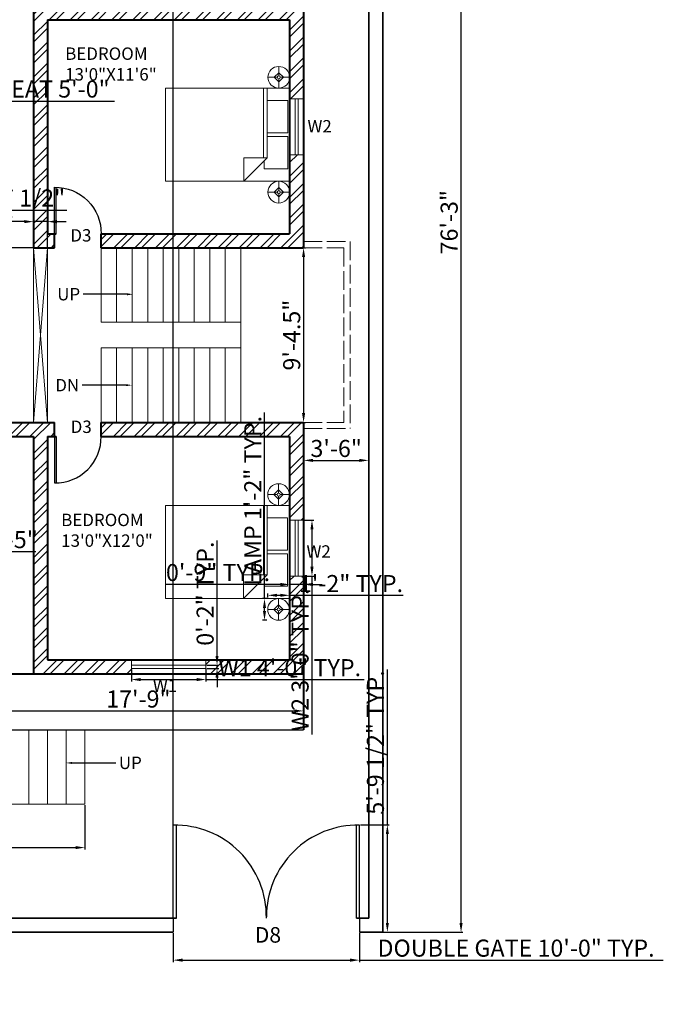
# Model space of a CAD drawing. Units: inches. Extents: x 2069 to 3028, y 691 to 1726.
# Tile 6 of 10: x 2613 to 3028, y 691 to 1325. Entities that reach past the tile are written whole.
import ezdxf
from ezdxf import colors
from ezdxf.entities.mleader import LeaderData, LeaderLine
from ezdxf.math import Vec2, Vec3

# ---------------------------------------------------------------- set-up
doc = ezdxf.new("R2010")
doc.units = ezdxf.units.IN
doc.linetypes.add('ACAD_ISO02W100', pattern=[15, 12, -3])
for name, color, linetype, lineweight in [('A-ANNO-DIMS', 2, 'Continuous', 18), ('A-DOOR', 3, 'Continuous', 25), ('A-FLOR', 7, 'Continuous', 25), ('A-FLOR-STRS', 7, 'Continuous', 20), ('A-FLOR-STRS-OVHD', 8, 'ACAD_ISO02W100', 18), ('A-FURN', 8, 'Continuous', 18), ('A-GLAZ', 4, 'Continuous', 20), ('A-WALL', 7, 'Continuous', 40), ('L-SITE-GATE', 3, 'Continuous', 25), ('L-SITE-WALL', 7, 'Continuous', 35)]:
    doc.layers.add(name, color=color, linetype=linetype, lineweight=lineweight)
for name, color, linetype, lineweight, true_color in [('A-ANNO-TEXT', 11, 'Continuous', 18, 0xf27172), ('A-AREA-IDEN', 11, 'Continuous', 25, 0xf27172), ('A-WALL-OPEN', 143, 'Continuous', 20, 0x7aafdf), ('A-WALL-PATT', 143, 'Continuous', 13, 0x7aafdf)]:
    doc.layers.add(name, color=color, linetype=linetype, lineweight=lineweight, true_color=true_color)
doc.styles.get("Standard").update_dxf_attribs({"font": 'arial.ttf'})
doc.dimstyles.new('ISO-25', dxfattribs={"dimtxt": 11, "dimasz": 6, "dimexe": 1.25, "dimexo": 0.625, "dimtad": 1, "dimlunit": 3, "dimtxsty": 'Standard', "dimcen": 2.5, "dimclrd": 3, "dimclre": 5, "dimclrt": 6, "dimadec": 0, "dimazin": 0, "dimtfac": 1, "dimtmove": 0, "dimatfit": 3, "dimfxl": 1, "dimarcsym": 0})

# ---------------------------------------------------------------- blocks, each defined once
blk = doc.blocks.new('Bed - Queen')
for p, q in [((0, -80.00003), (0, 0)), ((0, 0), (59.99999, 0)), ((59.99999, 0), (59.99999, -80.00003)), ((7.99999, -1.2), (28.79998, -1.2)), ((7.99999, -14.4), (7.99999, -1.2)), ((28.79998, -1.2), (28.79998, -14.4)), ((31.19999, -1.2), (51.99999, -1.2)), ((31.19999, -14.4), (31.19999, -1.2)), ((51.99999, -1.2), (51.99999, -16.4)), ((0, -14.4), (44.8, -14.4)), ((44.8, -16.8), (0, -16.8)), ((59.99999, -29.6), (44.8, -14.4)), ((44.8, -14.4), (44.8, -29.6)), ((51.99999, -16.4), (46.79936, -16.4)), ((44.8, -29.6), (59.99999, -29.6)), ((59.99999, -80.00003), (0, -80.00003))]:
    blk.add_line(p, q)
blk = doc.blocks.new('Lamp - Table')
for p, q in [((0, 7), (0, 1)), ((-1, 0), (-7, 0)), ((0, 3), (-3, 0)), ((-3, 0), (0, -3)), ((3, 0), (0, 3)), ((0, -3), (3, 0)), ((1, 0), (7, 0)), ((0, -1), (0, -7))]:
    blk.add_line(p, q)
for radius in [7, 1]:
    blk.add_circle((0, 0), radius)
blk = doc.blocks.new('*D26')
at = {"layer": 'A-ANNO-DIMS', "color": 0, "lineweight": -2, "transparency": 16777216}
for p, q in [((2796.58, 1178.39), (2797.2, 1178.39)), ((2795.95, 1172.39), (2795.95, 1071.89)), ((2796.58, 1065.89), (2797.2, 1065.89))]:
    blk.add_line(p, q, dxfattribs=at)
at = {"layer": 'A-ANNO-DIMS', "color": 0, "transparency": 16777216}
for points in [[(2794.95, 1172.39), (2796.95, 1172.39), (2795.95, 1178.39)], [(2794.95, 1071.89), (2796.95, 1071.89), (2795.95, 1065.89)]]:
    blk.add_solid(points, dxfattribs=at)
at = {"layer": 'Defpoints', "color": 0, "transparency": 16777216}
for p in [(2795.95, 1178.39), (2795.95, 1065.89), (2795.95, 1065.89)]:
    blk.add_point(p, dxfattribs=at)
at = {"layer": 'A-ANNO-DIMS', "color": 0, "transparency": 16777216, "insert": (2789.71, 1122.14), "char_height": 11, "attachment_point": 5, "rotation": 90}
blk.add_mtext('9\'-4.5"', dxfattribs=at)
blk = doc.blocks.new('*D27')
at = {"layer": 'A-ANNO-DIMS', "color": 0, "lineweight": -2, "transparency": 16777216}
for p, q in [((2795.95, 1060.76), (2795.95, 1040.17)), ((2837.95, 1060.76), (2837.95, 1040.17)), ((2801.95, 1041.42), (2831.95, 1041.42))]:
    blk.add_line(p, q, dxfattribs=at)
at = {"layer": 'A-ANNO-DIMS', "color": 0, "transparency": 16777216}
for points in [[(2801.95, 1042.42), (2801.95, 1040.42), (2795.95, 1041.42)], [(2831.95, 1042.42), (2831.95, 1040.42), (2837.95, 1041.42)]]:
    blk.add_solid(points, dxfattribs=at)
at = {"layer": 'Defpoints', "color": 0, "transparency": 16777216}
for p in [(2795.95, 1061.39), (2837.95, 1061.39), (2837.95, 1041.42)]:
    blk.add_point(p, dxfattribs=at)
at = {"layer": 'A-ANNO-DIMS', "color": 0, "transparency": 16777216, "insert": (2816.95, 1047.67), "char_height": 11, "attachment_point": 5}
blk.add_mtext('3\'-6"', dxfattribs=at)
blk = doc.blocks.new('*D28')
at = {"layer": 'A-ANNO-DIMS', "color": 0, "lineweight": -2, "transparency": 16777216}
for p, q in [((2582.95, 868.51), (2582.95, 881.23)), ((2588.95, 879.98), (2789.95, 879.98)), ((2795.95, 868.51), (2795.95, 881.23))]:
    blk.add_line(p, q, dxfattribs=at)
at = {"layer": 'A-ANNO-DIMS', "color": 0, "transparency": 16777216}
for points in [[(2588.95, 880.98), (2588.95, 878.98), (2582.95, 879.98)], [(2789.95, 880.98), (2789.95, 878.98), (2795.95, 879.98)]]:
    blk.add_solid(points, dxfattribs=at)
at = {"layer": 'Defpoints', "color": 0, "transparency": 16777216}
for p in [(2795.95, 879.98), (2582.95, 867.89), (2795.95, 867.89)]:
    blk.add_point(p, dxfattribs=at)
at = {"layer": 'A-ANNO-DIMS', "color": 0, "transparency": 16777216, "insert": (2689.45, 886.22), "char_height": 11, "attachment_point": 5}
blk.add_mtext('17\'-9"', dxfattribs=at)
blk = doc.blocks.new('*D32')
at = {"layer": 'A-ANNO-DIMS', "color": 0, "lineweight": -2, "transparency": 16777216}
for p, q in [((2438.95, 819.26), (2438.95, 790.68)), ((2654.95, 819.26), (2654.95, 790.68)), ((2444.95, 791.93), (2648.95, 791.93))]:
    blk.add_line(p, q, dxfattribs=at)
at = {"layer": 'A-ANNO-DIMS', "color": 0, "transparency": 16777216}
for points in [[(2444.95, 792.93), (2444.95, 790.93), (2438.95, 791.93)], [(2648.95, 792.93), (2648.95, 790.93), (2654.95, 791.93)]]:
    blk.add_solid(points, dxfattribs=at)
at = {"layer": 'Defpoints', "color": 0, "transparency": 16777216}
for p in [(2438.95, 819.89), (2654.95, 819.89), (2654.95, 791.93)]:
    blk.add_point(p, dxfattribs=at)
at = {"layer": 'A-ANNO-DIMS', "color": 0, "transparency": 16777216, "insert": (2546.95, 798.17), "char_height": 11, "attachment_point": 5}
blk.add_mtext("18'", dxfattribs=at)
blk = doc.blocks.new('GATE-DOUBLE-120IN')
for p, q in [((0, 0), (0, 60)), ((2, 0), (2, 60)), ((118, 0), (118, 60)), ((120, 0), (120, 60)), ((0, 0), (0, -9)), ((120, 0), (120, -9))]:
    blk.add_line(p, q)
for centre, radius, start, end in [((1, 1), 59.01, 359.02898, 90.97102), ((119, 1.02), 58.99, 89.0287, 180.01646)]:
    blk.add_arc(centre, radius, start, end)
blk = doc.blocks.new('DOOR-SWING-30IN')
for p, q in [((-1, 0), (-1, 30)), ((0, 0), (0, 30))]:
    blk.add_line(p, q)
blk.add_arc((-0.5, 0.5), 29.5, 89.02898, 180.97102)
blk = doc.blocks.new('WINDOW-36IN')
for p, q in [((0, 0), (9, 0)), ((3.5, 0), (3.5, -36)), ((5.5, 0), (5.5, -36)), ((0, -36), (9, -36))]:
    blk.add_line(p, q)
blk = doc.blocks.new('CASED-OPENING-112_5IN')
for p, q in [((9, 0), (0, -112.5)), ((9, -112.5), (0, 0)), ((0, 0), (0, -112.5)), ((9, 0), (9, -112.5))]:
    blk.add_line(p, q)
blk = doc.blocks.new('WINDOW-SASH-48IN')
for p, q in [((0, 0), (48, 0)), ((0, -2), (48, -2))]:
    blk.add_line(p, q)
blk = doc.blocks.new('*D48')
at = {"layer": 'A-ANNO-DIMS', "color": 5, "lineweight": -2, "transparency": 16777216}
for p, q in [((2485.97, 1196.86), (2485.97, 1203.98)), ((2529.25, 1196.86), (2529.25, 1203.98))]:
    blk.add_line(p, q, dxfattribs=at)
at = {"layer": 'A-ANNO-DIMS', "color": 3, "lineweight": -2, "transparency": 16777216}
for p, q in [((2491.97, 1202.73), (2523.25, 1202.73)), ((2529.25, 1202.73), (2643.33, 1202.73))]:
    blk.add_line(p, q, dxfattribs=at)
at = {"layer": 'A-ANNO-DIMS', "color": 3, "transparency": 16777216}
for points in [[(2491.97, 1203.73), (2491.97, 1201.73), (2485.97, 1202.73)], [(2523.25, 1203.73), (2523.25, 1201.73), (2529.25, 1202.73)]]:
    blk.add_solid(points, dxfattribs=at)
at = {"layer": 'Defpoints', "color": 0, "transparency": 16777216}
for p in [(2529.25, 1202.73), (2485.97, 1196.23), (2529.25, 1196.23)]:
    blk.add_point(p, dxfattribs=at)
at = {"layer": 'A-ANNO-DIMS', "color": 6, "transparency": 16777216, "insert": (2589.29, 1209.04), "char_height": 11, "attachment_point": 5}
blk.add_mtext('CHAIR 3\'-7 1/2"', dxfattribs=at)
blk = doc.blocks.new('*D50')
at = {"layer": 'A-ANNO-DIMS', "color": 3, "lineweight": -2, "transparency": 16777216}
for p, q in [((2770.76, 952.37), (2770.76, 1072.3)), ((2770.76, 944.37), (2770.76, 946.37))]:
    blk.add_line(p, q, dxfattribs=at)
at = {"layer": 'A-ANNO-DIMS', "color": 5, "lineweight": -2, "transparency": 16777216}
for p, q in [((2772.24, 952.37), (2769.51, 952.37)), ((2772.24, 938.37), (2769.51, 938.37))]:
    blk.add_line(p, q, dxfattribs=at)
at = {"layer": 'A-ANNO-DIMS', "color": 3, "transparency": 16777216}
for points in [[(2769.76, 946.37), (2771.76, 946.37), (2770.76, 952.37)], [(2769.76, 944.37), (2771.76, 944.37), (2770.76, 938.37)]]:
    blk.add_solid(points, dxfattribs=at)
at = {"layer": 'Defpoints', "color": 0, "transparency": 16777216}
for p in [(2770.76, 952.37), (2772.86, 952.37), (2772.86, 938.37)]:
    blk.add_point(p, dxfattribs=at)
at = {"layer": 'A-ANNO-DIMS', "color": 6, "transparency": 16777216, "insert": (2764.61, 1015.34), "char_height": 11, "attachment_point": 5, "rotation": 90}
blk.add_mtext('LAMP 1\'-2" TYP.', dxfattribs=at)
blk = doc.blocks.new('*D51')
at = {"layer": 'A-ANNO-DIMS', "color": 5, "lineweight": -2, "transparency": 16777216}
for p, q in [((2772.86, 953), (2772.86, 955.72)), ((2786.86, 953), (2786.86, 955.72))]:
    blk.add_line(p, q, dxfattribs=at)
at = {"layer": 'A-ANNO-DIMS', "color": 3, "lineweight": -2, "transparency": 16777216}
for p, q in [((2778.86, 954.47), (2780.86, 954.47)), ((2786.86, 954.47), (2860.13, 954.47))]:
    blk.add_line(p, q, dxfattribs=at)
at = {"layer": 'A-ANNO-DIMS', "color": 3, "transparency": 16777216}
for points in [[(2778.86, 955.47), (2778.86, 953.47), (2772.86, 954.47)], [(2780.86, 955.47), (2780.86, 953.47), (2786.86, 954.47)]]:
    blk.add_solid(points, dxfattribs=at)
at = {"layer": 'Defpoints', "color": 0, "transparency": 16777216}
for p in [(2772.86, 952.37), (2786.86, 954.47), (2786.86, 952.37)]:
    blk.add_point(p, dxfattribs=at)
at = {"layer": 'A-ANNO-DIMS', "color": 6, "transparency": 16777216, "insert": (2826.5, 960.62), "char_height": 11, "attachment_point": 5}
blk.add_mtext('1\'-2" TYP.', dxfattribs=at)
blk = doc.blocks.new('*D52')
at = {"layer": 'A-ANNO-DIMS', "color": 5, "lineweight": -2, "transparency": 16777216}
for p, q in [((2796.58, 1002.89), (2802.6, 1002.89)), ((2796.58, 966.89), (2802.6, 966.89))]:
    blk.add_line(p, q, dxfattribs=at)
at = {"layer": 'A-ANNO-DIMS', "color": 3, "lineweight": -2, "transparency": 16777216}
for p, q in [((2801.35, 996.89), (2801.35, 972.89)), ((2801.35, 966.89), (2801.35, 864.82))]:
    blk.add_line(p, q, dxfattribs=at)
at = {"layer": 'A-ANNO-DIMS', "color": 3, "transparency": 16777216}
for points in [[(2800.35, 996.89), (2802.35, 996.89), (2801.35, 1002.89)], [(2800.35, 972.89), (2802.35, 972.89), (2801.35, 966.89)]]:
    blk.add_solid(points, dxfattribs=at)
at = {"layer": 'Defpoints', "color": 0, "transparency": 16777216}
for p in [(2795.95, 1002.89), (2795.95, 966.89), (2801.35, 966.89)]:
    blk.add_point(p, dxfattribs=at)
at = {"layer": 'A-ANNO-DIMS', "color": 6, "transparency": 16777216, "insert": (2795.11, 912.85), "char_height": 11, "attachment_point": 5, "rotation": 90}
blk.add_mtext('W2 3\'-0" TYP.', dxfattribs=at)
blk = doc.blocks.new('*D53')
at = {"layer": 'A-ANNO-DIMS', "color": 5, "lineweight": -2, "transparency": 16777216}
for p, q in [((2786.95, 966.26), (2786.95, 960.24)), ((2795.95, 966.26), (2795.95, 960.24))]:
    blk.add_line(p, q, dxfattribs=at)
at = {"layer": 'A-ANNO-DIMS', "color": 3, "lineweight": -2, "transparency": 16777216}
for p, q in [((2780.95, 961.49), (2706.65, 961.49)), ((2795.95, 961.49), (2786.95, 961.49)), ((2801.95, 961.49), (2807.95, 961.49))]:
    blk.add_line(p, q, dxfattribs=at)
at = {"layer": 'A-ANNO-DIMS', "color": 3, "transparency": 16777216}
for points in [[(2780.95, 962.49), (2780.95, 960.49), (2786.95, 961.49)], [(2801.95, 962.49), (2801.95, 960.49), (2795.95, 961.49)]]:
    blk.add_solid(points, dxfattribs=at)
at = {"layer": 'Defpoints', "color": 0, "transparency": 16777216}
for p in [(2786.95, 966.89), (2795.95, 966.89), (2786.95, 961.49)]:
    blk.add_point(p, dxfattribs=at)
at = {"layer": 'A-ANNO-DIMS', "color": 6, "transparency": 16777216, "insert": (2740.8, 967.73), "char_height": 11, "attachment_point": 5}
blk.add_mtext('0\'-9" TYP.', dxfattribs=at)
blk = doc.blocks.new('*D58')
at = {"layer": 'A-ANNO-DIMS', "color": 5, "lineweight": -2, "transparency": 16777216}
for p, q in [((2684.95, 906.76), (2684.95, 898.94)), ((2732.95, 906.76), (2732.95, 898.94))]:
    blk.add_line(p, q, dxfattribs=at)
at = {"layer": 'A-ANNO-DIMS', "color": 3, "lineweight": -2, "transparency": 16777216}
for p, q in [((2690.95, 900.19), (2726.95, 900.19)), ((2732.95, 900.19), (2835.02, 900.19))]:
    blk.add_line(p, q, dxfattribs=at)
at = {"layer": 'A-ANNO-DIMS', "color": 3, "transparency": 16777216}
for points in [[(2690.95, 901.19), (2690.95, 899.19), (2684.95, 900.19)], [(2726.95, 901.19), (2726.95, 899.19), (2732.95, 900.19)]]:
    blk.add_solid(points, dxfattribs=at)
at = {"layer": 'Defpoints', "color": 0, "transparency": 16777216}
for p in [(2684.95, 907.39), (2732.95, 907.39), (2732.95, 900.19)]:
    blk.add_point(p, dxfattribs=at)
at = {"layer": 'A-ANNO-DIMS', "color": 6, "transparency": 16777216, "insert": (2786.99, 906.43), "char_height": 11, "attachment_point": 5}
blk.add_mtext('W1 4\'-0" TYP.', dxfattribs=at)
blk = doc.blocks.new('*D59')
at = {"layer": 'A-ANNO-DIMS', "color": 3, "lineweight": -2, "transparency": 16777216}
for p, q in [((2740.15, 915.39), (2740.15, 989.69)), ((2740.15, 907.39), (2740.15, 909.39)), ((2740.15, 901.39), (2740.15, 895.39))]:
    blk.add_line(p, q, dxfattribs=at)
at = {"layer": 'A-ANNO-DIMS', "color": 5, "lineweight": -2, "transparency": 16777216}
for p, q in [((2733.58, 909.39), (2741.4, 909.39)), ((2733.58, 907.39), (2741.4, 907.39))]:
    blk.add_line(p, q, dxfattribs=at)
at = {"layer": 'A-ANNO-DIMS', "color": 3, "transparency": 16777216}
for points in [[(2739.15, 915.39), (2741.15, 915.39), (2740.15, 909.39)], [(2739.15, 901.39), (2741.15, 901.39), (2740.15, 907.39)]]:
    blk.add_solid(points, dxfattribs=at)
at = {"layer": 'Defpoints', "color": 0, "transparency": 16777216}
for p in [(2732.95, 909.39), (2732.95, 907.39), (2740.15, 909.39)]:
    blk.add_point(p, dxfattribs=at)
at = {"layer": 'A-ANNO-DIMS', "color": 6, "transparency": 16777216, "insert": (2733.91, 955.54), "char_height": 11, "attachment_point": 5, "rotation": 90}
blk.add_mtext('0\'-2" TYP.', dxfattribs=at)
blk = doc.blocks.new('*D67')
at = {"layer": 'A-ANNO-DIMS', "color": 5, "lineweight": -2, "transparency": 16777216}
for p, q in [((2557.52, 986.45), (2557.52, 981.45)), ((2586.69, 986.45), (2586.69, 981.45))]:
    blk.add_line(p, q, dxfattribs=at)
at = {"layer": 'A-ANNO-DIMS', "color": 3, "lineweight": -2, "transparency": 16777216}
for p, q in [((2563.52, 982.7), (2580.69, 982.7)), ((2586.69, 982.7), (2623.36, 982.7))]:
    blk.add_line(p, q, dxfattribs=at)
at = {"layer": 'A-ANNO-DIMS', "color": 3, "transparency": 16777216}
for points in [[(2563.52, 983.7), (2563.52, 981.7), (2557.52, 982.7)], [(2580.69, 983.7), (2580.69, 981.7), (2586.69, 982.7)]]:
    blk.add_solid(points, dxfattribs=at)
at = {"layer": 'Defpoints', "color": 0, "transparency": 16777216}
for p in [(2557.52, 987.08), (2586.69, 987.08), (2586.69, 982.7)]:
    blk.add_point(p, dxfattribs=at)
at = {"layer": 'A-ANNO-DIMS', "color": 6, "transparency": 16777216, "insert": (2608.03, 988.95), "char_height": 11, "attachment_point": 5}
blk.add_mtext('2\'-5"', dxfattribs=at)
blk = doc.blocks.new('*D70')
at = {"layer": 'A-ANNO-DIMS', "color": 5, "lineweight": -2, "transparency": 16777216}
for p, q in [((2711.95, 736.76), (2711.95, 718.14)), ((2831.95, 736.76), (2831.95, 718.14))]:
    blk.add_line(p, q, dxfattribs=at)
at = {"layer": 'A-ANNO-DIMS', "color": 3, "lineweight": -2, "transparency": 16777216}
for p, q in [((2717.95, 719.39), (2825.95, 719.39)), ((2831.95, 719.39), (3027.82, 719.39))]:
    blk.add_line(p, q, dxfattribs=at)
at = {"layer": 'A-ANNO-DIMS', "color": 3, "transparency": 16777216}
for points in [[(2717.95, 720.39), (2717.95, 718.39), (2711.95, 719.39)], [(2825.95, 720.39), (2825.95, 718.39), (2831.95, 719.39)]]:
    blk.add_solid(points, dxfattribs=at)
at = {"layer": 'Defpoints', "color": 0, "transparency": 16777216}
for p in [(2711.95, 737.39), (2831.95, 737.39), (2831.95, 719.39)]:
    blk.add_point(p, dxfattribs=at)
at = {"layer": 'A-ANNO-DIMS', "color": 6, "transparency": 16777216, "insert": (2932.89, 725.7), "char_height": 11, "attachment_point": 5}
blk.add_mtext('DOUBLE GATE 10\'-0" TYP.', dxfattribs=at)
blk = doc.blocks.new('*D71')
at = {"layer": 'A-ANNO-DIMS', "color": 3, "lineweight": -2, "transparency": 16777216}
for p, q in [((2849.95, 806.66), (2849.95, 906.59)), ((2849.95, 743.39), (2849.95, 800.66))]:
    blk.add_line(p, q, dxfattribs=at)
at = {"layer": 'A-ANNO-DIMS', "color": 5, "lineweight": -2, "transparency": 16777216}
for p, q in [((2832.58, 806.66), (2851.2, 806.66)), ((2832.58, 737.39), (2851.2, 737.39))]:
    blk.add_line(p, q, dxfattribs=at)
at = {"layer": 'A-ANNO-DIMS', "color": 3, "transparency": 16777216}
for points in [[(2848.95, 800.66), (2850.95, 800.66), (2849.95, 806.66)], [(2848.95, 743.39), (2850.95, 743.39), (2849.95, 737.39)]]:
    blk.add_solid(points, dxfattribs=at)
at = {"layer": 'Defpoints', "color": 0, "transparency": 16777216}
for p in [(2831.95, 806.66), (2849.95, 806.66), (2831.95, 737.39)]:
    blk.add_point(p, dxfattribs=at)
at = {"layer": 'A-ANNO-DIMS', "color": 6, "transparency": 16777216, "insert": (2843.64, 859.62), "char_height": 11, "attachment_point": 5, "rotation": 90}
blk.add_mtext('5\'-9 1/2" TYP.', dxfattribs=at)
blk = doc.blocks.new('*D72')
at = {"layer": 'A-ANNO-DIMS', "color": 5, "lineweight": -2, "transparency": 16777216}
for p, q in [((2621.33, 1178.39), (2603.83, 1178.39)), ((2621.33, 1065.89), (2603.83, 1065.89))]:
    blk.add_line(p, q, dxfattribs=at)
at = {"layer": 'A-ANNO-DIMS', "color": 3, "lineweight": -2, "transparency": 16777216}
for p, q in [((2605.08, 1172.39), (2605.08, 1071.89)), ((2605.08, 1065.89), (2605.08, 833.73))]:
    blk.add_line(p, q, dxfattribs=at)
at = {"layer": 'A-ANNO-DIMS', "color": 3, "transparency": 16777216}
for points in [[(2604.08, 1172.39), (2606.08, 1172.39), (2605.08, 1178.39)], [(2604.08, 1071.89), (2606.08, 1071.89), (2605.08, 1065.89)]]:
    blk.add_solid(points, dxfattribs=at)
at = {"layer": 'Defpoints', "color": 0, "transparency": 16777216}
for p in [(2621.95, 1178.39), (2605.08, 1065.89), (2621.95, 1065.89)]:
    blk.add_point(p, dxfattribs=at)
at = {"layer": 'A-ANNO-DIMS', "color": 6, "transparency": 16777216, "insert": (2598.76, 946.81), "char_height": 11, "attachment_point": 5, "rotation": 90}
blk.add_mtext('CASED OPENING 9\'-4 1/2" TYP.', dxfattribs=at)
blk = doc.blocks.new('*D73')
at = {"layer": 'A-ANNO-DIMS', "color": 3, "lineweight": -2, "transparency": 16777216}
for p, q in [((2615.95, 1195.26), (2541.65, 1195.26)), ((2630.95, 1195.26), (2621.95, 1195.26)), ((2636.95, 1195.26), (2642.95, 1195.26))]:
    blk.add_line(p, q, dxfattribs=at)
at = {"layer": 'A-ANNO-DIMS', "color": 5, "lineweight": -2, "transparency": 16777216}
for p, q in [((2621.95, 1179.01), (2621.95, 1196.51)), ((2630.95, 1179.01), (2630.95, 1196.51))]:
    blk.add_line(p, q, dxfattribs=at)
at = {"layer": 'A-ANNO-DIMS', "color": 3, "transparency": 16777216}
for points in [[(2615.95, 1196.26), (2615.95, 1194.26), (2621.95, 1195.26)], [(2636.95, 1196.26), (2636.95, 1194.26), (2630.95, 1195.26)]]:
    blk.add_solid(points, dxfattribs=at)
at = {"layer": 'Defpoints', "color": 0, "transparency": 16777216}
for p in [(2621.95, 1195.26), (2621.95, 1178.39), (2630.95, 1178.39)]:
    blk.add_point(p, dxfattribs=at)
at = {"layer": 'A-ANNO-DIMS', "color": 6, "transparency": 16777216, "insert": (2575.8, 1201.5), "char_height": 11, "attachment_point": 5}
blk.add_mtext('0\'-9" TYP.', dxfattribs=at)
blk = doc.blocks.new('*D80')
at = {"layer": 'A-ANNO-DIMS', "color": 5, "lineweight": -2, "transparency": 16777216}
for p, q in [((2492.66, 1281.34), (2492.66, 1271.71)), ((2552.66, 1281.34), (2552.66, 1271.71))]:
    blk.add_line(p, q, dxfattribs=at)
at = {"layer": 'A-ANNO-DIMS', "color": 3, "lineweight": -2, "transparency": 16777216}
for p, q in [((2498.66, 1272.96), (2546.66, 1272.96)), ((2552.66, 1272.96), (2674.06, 1272.96))]:
    blk.add_line(p, q, dxfattribs=at)
at = {"layer": 'A-ANNO-DIMS', "color": 3, "transparency": 16777216}
for points in [[(2498.66, 1273.96), (2498.66, 1271.96), (2492.66, 1272.96)], [(2546.66, 1273.96), (2546.66, 1271.96), (2552.66, 1272.96)]]:
    blk.add_solid(points, dxfattribs=at)
at = {"layer": 'Defpoints', "color": 0, "transparency": 16777216}
for p in [(2492.66, 1281.96), (2552.66, 1281.96), (2552.66, 1272.96)]:
    blk.add_point(p, dxfattribs=at)
at = {"layer": 'A-ANNO-DIMS', "color": 6, "transparency": 16777216, "insert": (2616.36, 1279.28), "char_height": 11, "attachment_point": 5}
blk.add_mtext('LOVESEAT 5\'-0"', dxfattribs=at)
blk = doc.blocks.new('*D86')
at = {"layer": 'A-ANNO-DIMS', "color": 5, "lineweight": -2, "transparency": 16777216}
for p, q in [((2847.58, 1652.39), (2898.7, 1652.39)), ((2847.58, 737.39), (2898.7, 737.39))]:
    blk.add_line(p, q, dxfattribs=at)
at = {"layer": 'A-ANNO-DIMS', "color": 3, "lineweight": -2, "transparency": 16777216}
blk.add_line((2897.45, 743.39), (2897.45, 1646.39), dxfattribs=at)
at = {"layer": 'A-ANNO-DIMS', "color": 3, "transparency": 16777216}
for points in [[(2896.45, 1646.39), (2898.45, 1646.39), (2897.45, 1652.39)], [(2896.45, 743.39), (2898.45, 743.39), (2897.45, 737.39)]]:
    blk.add_solid(points, dxfattribs=at)
at = {"layer": 'Defpoints', "color": 0, "transparency": 16777216}
for p in [(2846.95, 1652.39), (2897.45, 1652.39), (2846.95, 737.39)]:
    blk.add_point(p, dxfattribs=at)
at = {"layer": 'A-ANNO-DIMS', "color": 6, "transparency": 16777216, "insert": (2891.21, 1194.89), "char_height": 11, "attachment_point": 5, "rotation": 90}
blk.add_mtext('76\'-3"', dxfattribs=at)
blk = doc.blocks.new('*D89')
at = {"layer": 'A-ANNO-DIMS', "color": 5, "lineweight": -2, "transparency": 16777216}
for p, q in [((2336.92, 747.01), (2336.92, 1704.14)), ((2711.95, 747.01), (2711.95, 1704.14))]:
    blk.add_line(p, q, dxfattribs=at)
at = {"layer": 'A-ANNO-DIMS', "color": 3, "lineweight": -2, "transparency": 16777216}
blk.add_line((2342.92, 1702.89), (2705.95, 1702.89), dxfattribs=at)
at = {"layer": 'A-ANNO-DIMS', "color": 3, "transparency": 16777216}
for points in [[(2342.92, 1703.89), (2342.92, 1701.89), (2336.92, 1702.89)], [(2705.95, 1703.89), (2705.95, 1701.89), (2711.95, 1702.89)]]:
    blk.add_solid(points, dxfattribs=at)
at = {"layer": 'Defpoints', "color": 0, "transparency": 16777216}
for p in [(2711.95, 1702.89), (2336.92, 746.39), (2711.95, 746.39)]:
    blk.add_point(p, dxfattribs=at)
at = {"layer": 'A-ANNO-DIMS', "color": 6, "transparency": 16777216, "insert": (2524.44, 1709.13), "char_height": 11, "attachment_point": 5}
blk.add_mtext('31\'-3"', dxfattribs=at)

msp = doc.modelspace()

# ---------------------------------------------------------------- hatches: boundary and pattern name
at = {"layer": 'A-WALL-PATT'}
h = msp.add_hatch(dxfattribs=at)
h.set_pattern_fill('ANSI32', color=256)
h.paths.add_polyline_path([(2675.951, 1487.387), (2576.951, 1487.387), (2576.951, 1478.387), (2621.951, 1478.387), (2621.951, 1365.287), (2630.951, 1365.287), (2630.951, 1478.387), (2675.951, 1478.387)])
h.paths.add_polyline_path([(2765.951, 1487.387), (2711.951, 1487.387), (2711.951, 1478.387), (2756.951, 1478.387), (2756.951, 1424.387), (2765.951, 1424.387)])
h.paths.add_polyline_path([(2528.951, 1487.387), (2407.751, 1487.387), (2407.751, 1478.387), (2474.951, 1478.387), (2474.951, 1434.887), (2498.951, 1434.887), (2498.951, 1374.887), (2474.951, 1374.887), (2474.951, 1365.287), (2483.951, 1365.287), (2483.951, 1370.387), (2507.951, 1370.387), (2507.951, 1439.387), (2483.951, 1439.387), (2483.951, 1478.387), (2528.951, 1478.387)])
h.paths.add_polyline_path([(2374.151, 1487.387), (2297.951, 1487.387), (2297.951, 1424.387), (2306.951, 1424.387), (2306.951, 1478.387), (2374.151, 1478.387)])
h.paths.add_polyline_path([(2507.951, 1334.387), (2483.951, 1334.387), (2483.951, 1338.887), (2474.951, 1338.887), (2474.951, 1334.387), (2306.951, 1334.387), (2306.951, 1388.387), (2297.951, 1388.387), (2297.951, 1334.387), (2267.951, 1334.387), (2267.951, 1274.387), (2276.951, 1274.387), (2276.951, 1325.387), (2297.951, 1325.387), (2423.951, 1325.387), (2423.951, 1187.387), (2419.451, 1187.387), (2419.451, 1178.387), (2432.951, 1178.387), (2432.951, 1325.387), (2507.951, 1325.387)])
h.paths.add_polyline_path([(2795.951, 1334.387), (2630.951, 1334.387), (2630.951, 1338.887), (2621.951, 1338.887), (2621.951, 1178.387), (2635.451, 1178.387), (2635.451, 1187.387), (2630.951, 1187.387), (2630.951, 1325.387), (2786.951, 1325.387), (2786.951, 1274.387), (2795.951, 1274.387)])
h.paths.add_polyline_path([(2765.951, 1388.387), (2756.951, 1388.387), (2756.951, 1334.387), (2765.951, 1334.387)])
h.paths.add_polyline_path([(2795.951, 1238.387), (2786.951, 1238.387), (2786.951, 1187.387), (2665.451, 1187.387), (2665.451, 1178.387), (2795.951, 1178.387)], flags=17)
h.paths.add_polyline_path([(2389.451, 1187.387), (2276.951, 1187.387), (2276.951, 1238.387), (2267.951, 1238.387), (2267.951, 1178.387), (2297.951, 1178.387), (2297.951, 1173.287), (2307.451, 1173.287), (2307.451, 1178.387), (2389.451, 1178.387)])
h.paths.add_polyline_path([(2377.451, 1142.387), (2306.951, 1142.387), (2306.951, 1146.887), (2297.951, 1146.887), (2297.951, 1142.387), (2297.951, 1137.887), (2306.951, 1137.887), (2372.951, 1137.887), (2372.951, 1133.387), (2377.451, 1133.387)])
h.paths.add_polyline_path([(2795.951, 1065.887), (2665.451, 1065.887), (2665.451, 1056.887), (2786.951, 1056.887), (2786.951, 1002.887), (2795.951, 1002.887), (2795.951, 1056.887)])
h.paths.add_polyline_path([(2795.951, 966.887), (2786.951, 966.887), (2786.951, 912.887), (2732.951, 912.887), (2732.951, 903.887), (2795.951, 903.887)])
h.paths.add_polyline_path([(2483.951, 917.387), (2474.951, 917.387), (2474.951, 912.887), (2414.951, 912.887), (2414.951, 903.887), (2483.951, 903.887)])
h.paths.add_polyline_path([(2366.951, 912.887), (2306.951, 912.887), (2306.951, 960.887), (2297.951, 960.887), (2297.951, 903.887), (2366.951, 903.887)])
h.paths.add_polyline_path([(2498.951, 1056.887), (2498.951, 1065.887), (2377.451, 1065.887), (2377.451, 1111.787), (2372.951, 1111.787), (2372.951, 1065.887), (2306.951, 1065.887), (2306.951, 1116.287), (2297.951, 1116.287), (2297.951, 1056.887), (2297.951, 1008.887), (2306.951, 1008.887), (2306.951, 1056.887), (2474.951, 1056.887), (2474.951, 947.387), (2483.951, 947.387), (2483.951, 1056.887)])
h = msp.add_hatch(dxfattribs=at)
h.set_pattern_fill('ANSI32', color=256)
h.paths.add_polyline_path([(2684.951, 912.887), (2630.951, 912.887), (2630.951, 1056.887), (2635.451, 1056.887), (2635.451, 1065.887), (2606.951, 1065.887), (2606.951, 1056.887), (2621.951, 1056.887), (2621.951, 903.887), (2684.951, 903.887)])

# ---------------------------------------------------------------- linework, layer by layer
at = {"layer": 'A-FLOR'}
msp.add_line((2297.951, 867.887), (2795.951, 867.887), dxfattribs=at)
at = {"layer": 'A-FLOR-STRS'}
for p, q in [((2665.451, 1178.387), (2665.451, 1130.387)), ((2675.451, 1178.387), (2675.451, 1130.387)), ((2685.451, 1178.387), (2685.451, 1130.387)), ((2695.451, 1178.387), (2695.451, 1130.387)), ((2705.451, 1178.387), (2705.451, 1130.387)), ((2715.451, 1178.387), (2715.451, 1130.387)), ((2725.451, 1178.387), (2725.451, 1130.387)), ((2735.451, 1178.387), (2735.451, 1130.387)), ((2745.451, 1178.387), (2745.451, 1130.387)), ((2755.451, 1178.387), (2755.451, 1113.887)), ((2665.451, 1130.387), (2755.451, 1130.387)), ((2665.451, 1113.887), (2755.451, 1113.887)), ((2665.451, 1113.887), (2665.451, 1065.887)), ((2675.451, 1113.887), (2675.451, 1065.887)), ((2685.451, 1113.887), (2685.451, 1065.887)), ((2695.451, 1113.887), (2695.451, 1065.887)), ((2705.451, 1113.887), (2705.451, 1065.887)), ((2715.451, 1113.887), (2715.451, 1065.887)), ((2725.451, 1113.887), (2725.451, 1065.887)), ((2735.451, 1113.887), (2735.451, 1065.887)), ((2745.451, 1113.887), (2745.451, 1065.887)), ((2755.451, 1113.887), (2755.451, 1065.887)), ((2618.951, 819.887), (2618.951, 867.887)), ((2630.951, 819.887), (2630.951, 867.887)), ((2642.951, 819.887), (2642.951, 867.887)), ((2654.951, 819.887), (2654.951, 867.887)), ((2438.951, 819.887), (2654.951, 819.887))]:
    msp.add_line(p, q, dxfattribs=at)
at = {"layer": 'A-FLOR-STRS-OVHD'}
for p, q in [((2795.951, 1182.387), (2825.951, 1182.387)), ((2825.951, 1182.387), (2825.951, 1061.887)), ((2795.951, 1178.387), (2821.951, 1178.387)), ((2821.951, 1178.387), (2821.951, 1065.887)), ((2795.951, 1065.887), (2821.951, 1065.887)), ((2795.951, 1061.887), (2825.951, 1061.887))]:
    msp.add_line(p, q, dxfattribs=at)
at = {"layer": 'A-GLAZ'}
for p, q in [((2684.951, 912.887), (2684.951, 903.887)), ((2732.951, 912.887), (2732.951, 903.887))]:
    msp.add_line(p, q, dxfattribs=at)
at = {"layer": 'A-WALL'}
for p, q in [((2621.951, 1338.887), (2621.951, 1178.387)), ((2795.951, 1334.387), (2795.951, 1178.387)), ((2630.951, 1325.387), (2630.951, 1187.387)), ((2630.951, 1325.387), (2786.951, 1325.387)), ((2786.951, 1325.387), (2786.951, 1187.387)), ((2630.951, 1187.387), (2636.451, 1187.387)), ((2635.451, 1178.387), (2635.451, 1187.387)), ((2665.451, 1178.387), (2665.451, 1187.387)), ((2665.451, 1187.387), (2786.951, 1187.387)), ((2621.951, 1178.387), (2635.451, 1178.387)), ((2665.451, 1178.387), (2795.951, 1178.387)), ((2569.951, 1065.887), (2635.451, 1065.887)), ((2635.451, 1056.887), (2635.451, 1065.887)), ((2665.451, 1056.887), (2665.451, 1065.887)), ((2665.451, 1065.887), (2795.951, 1065.887)), ((2795.951, 1065.887), (2795.951, 1056.887)), ((2570.951, 1056.887), (2621.951, 1056.887)), ((2621.951, 1056.887), (2621.951, 903.887)), ((2630.951, 1056.887), (2630.951, 912.887)), ((2630.951, 1056.887), (2636.451, 1056.887)), ((2665.451, 1056.887), (2786.951, 1056.887)), ((2786.951, 1056.887), (2786.951, 912.887)), ((2795.951, 1056.887), (2795.951, 867.887)), ((2630.951, 912.887), (2786.951, 912.887)), ((2582.951, 903.887), (2795.951, 903.887))]:
    msp.add_line(p, q, dxfattribs=at)
at = {"layer": 'L-SITE-WALL'}
for p, q in [((2846.951, 1652.387), (2846.951, 737.387)), ((2837.951, 1643.387), (2837.951, 1178.387)), ((2837.951, 1178.387), (2837.951, 1065.887)), ((2837.951, 1065.887), (2837.951, 746.387)), ((2335.919, 746.387), (2713.951, 746.387)), ((2829.951, 746.387), (2837.951, 746.387)), ((2336.919, 737.387), (2711.951, 737.387)), ((2831.951, 737.387), (2846.951, 737.387))]:
    msp.add_line(p, q, dxfattribs=at)

# ---------------------------------------------------------------- block references
at = {"layer": 'A-DOOR', "extrusion": (0, 0, -1), "zscale": -1}
msp.add_blockref('DOOR-SWING-30IN', (-2635.451, 1187.387), dxfattribs=at)
at = {"layer": 'A-DOOR', "rotation": 180}
msp.add_blockref('DOOR-SWING-30IN', (2635.451, 1056.887), dxfattribs=at)
at = {"layer": 'A-FURN', "rotation": 270}
for name, p in [('Lamp - Table', (2779.951, 1288.251)), ('Bed - Queen', (2786.951, 1281.251)), ('Lamp - Table', (2779.863, 1019.372)), ('Bed - Queen', (2786.863, 1012.372))]:
    msp.add_blockref(name, p, dxfattribs=at)
at = {"layer": 'A-FURN', "xscale": -1, "rotation": 270}
for p in [(2779.951, 1214.251), (2779.863, 945.372)]:
    msp.add_blockref('Lamp - Table', p, dxfattribs=at)
at = {"layer": 'A-GLAZ'}
for name, p in [('WINDOW-36IN', (2786.951, 1274.387)), ('WINDOW-SASH-48IN', (2684.951, 909.387))]:
    msp.add_blockref(name, p, dxfattribs=at)
at = {"layer": 'A-GLAZ', "rotation": 180}
msp.add_blockref('WINDOW-36IN', (2795.951, 966.887), dxfattribs=at)
at = {"layer": 'A-WALL-OPEN', "rotation": 180}
msp.add_blockref('CASED-OPENING-112_5IN', (2630.951, 1065.887), dxfattribs=at)
at = {"layer": 'L-SITE-GATE'}
msp.add_blockref('GATE-DOUBLE-120IN', (2711.951, 746.387), dxfattribs=at)

# ---------------------------------------------------------------- texts
at = {"layer": 'A-ANNO-TEXT', "attachment_point": 1}
for s, insert, char_height in [('{\\fArial|b1|i0|c0|p34;W2}', (2798.476, 1260.708), 8), ('{\\fArial|b1|i0|c0|p34;D3}', (2645.612, 1190.405), 8), ('{\\fArial|b1|i0|c0|p34;D3}', (2645.821, 1067.079), 8), ('{\\fArial|b1|i0|c0|p34;W2}', (2797.827, 986.701), 8), ('{\\fArial|b1|i0|c0|p34;W1}', (2698.804, 900.263), 8), ('{\\fArial|b1|i0|c0|p34;D8}', (2764.492, 740.659), 10)]:
    msp.add_mtext_dynamic_manual_height_columns(s, width=34.05605, gutter_width=12.5, heights=[0], dxfattribs=dict(at, insert=insert, char_height=char_height))
at = {"layer": 'A-AREA-IDEN', "char_height": 8, "attachment_point": 1}
for s, insert in [('BEDROOM\\P13\'0"X11\'6"', (2642.274, 1307.498)), ('BEDROOM\\P13\'0"X12\'0"', (2639.712, 1007.048))]:
    msp.add_mtext_dynamic_manual_height_columns(s, width=119.20948, gutter_width=12.5, heights=[0], dxfattribs=dict(at, insert=insert))

# ---------------------------------------------------------------- dimensions: what is measured, and where the dimension line sits
at = {"layer": 'A-ANNO-DIMS'}
for base, p1, p2, override, picture, middle in [((2711.951, 1702.887), (2336.919, 746.387), (2711.951, 746.387), {"dimdec": 1, "dimlfac": 1, "dimrnd": 0, "dimzin": 1, "dimdsep": 46, "dimlunit": 4, "dimfrac": 2}, '*D89', (2524.435, 1709.132)), ((2837.951, 1041.422), (2795.951, 1061.387), (2837.951, 1061.387), {"dimclrd": 0, "dimclre": 0, "dimclrt": 0}, '*D27', (2816.951, 1047.667)), ((2586.686, 982.704), (2557.517, 987.079), (2586.686, 987.079), {"dimdec": 1, "dimlfac": 1, "dimrnd": 0, "dimzin": 1, "dimdsep": 46, "dimlunit": 4, "dimfrac": 2}, '*D67', (2608.025, 988.945)), ((2795.951, 879.977), (2582.951, 867.887), (2795.951, 867.887), {"dimclrd": 0, "dimclre": 0, "dimclrt": 0}, '*D28', (2689.451, 886.219)), ((2654.951, 791.93), (2438.951, 819.887), (2654.951, 819.887), {"dimclrd": 0, "dimclre": 0, "dimclrt": 0}, '*D32', (2546.951, 798.172))]:
    dim = msp.add_linear_dim(base=base, p1=p1, p2=p2, dimstyle='ISO-25', override=override, dxfattribs=at)
    dim.commit()
    dim.dimension.update_dxf_attribs({"geometry": picture, "text_midpoint": middle})
for base, p1, p2, override, picture, middle in [((2897.451, 1652.387), (2846.951, 737.387), (2846.951, 1652.387), {"dimdec": 1, "dimlfac": 1, "dimrnd": 0, "dimzin": 1, "dimdsep": 46, "dimlunit": 4, "dimfrac": 2}, '*D86', (2891.206, 1194.887)), ((2795.951, 1065.887), (2795.951, 1178.387), (2795.951, 1065.887), {"dimclrd": 0, "dimclre": 0, "dimclrt": 0}, '*D26', (2789.71, 1122.137))]:
    dim = msp.add_linear_dim(base=base, p1=p1, p2=p2, angle=90, dimstyle='ISO-25', override=override, dxfattribs=at)
    dim.commit()
    dim.dimension.update_dxf_attribs({"geometry": picture, "text_midpoint": middle})
for base, p1, p2, text, picture, middle in [((2552.655, 1272.963), (2492.655, 1281.963), (2552.655, 1281.963), 'LOVESEAT <>', '*D80', (2616.359, 1279.28)), ((2529.253, 1202.727), (2485.968, 1196.234), (2529.253, 1196.234), 'CHAIR <>', '*D48', (2589.291, 1209.043)), ((2786.863, 954.472), (2772.863, 952.372), (2786.863, 952.372), '<> TYP.', '*D51', (2826.495, 960.623)), ((2732.951, 900.187), (2684.951, 907.387), (2732.951, 907.387), 'W1 <> TYP.', '*D58', (2786.987, 906.428)), ((2831.951, 719.387), (2711.951, 737.387), (2831.951, 737.387), 'DOUBLE GATE <> TYP.', '*D70', (2932.887, 725.703))]:
    dim = msp.add_linear_dim(base=base, p1=p1, p2=p2, text=text, dimstyle='ISO-25', override={"dimdec": 1, "dimlfac": 1, "dimrnd": 0, "dimzin": 1, "dimdsep": 46, "dimlunit": 4, "dimfrac": 2}, dxfattribs=at)
    dim.commit()
    dim.dimension.update_dxf_attribs({"geometry": picture, "text_midpoint": middle})
for base, p1, p2, angle, text, picture, middle in [((2621.951, 1195.262), (2630.951, 1178.387), (2621.951, 1178.387), 180, '<> TYP.', '*D73', (2575.801, 1201.503)), ((2605.076, 1065.887), (2621.951, 1178.387), (2621.951, 1065.887), 270, 'CASED OPENING <> TYP.', '*D72', (2598.76, 946.808)), ((2770.763, 952.372), (2772.863, 938.372), (2772.863, 952.372), 90, 'LAMP <> TYP.', '*D50', (2764.612, 1015.336)), ((2801.351, 966.887), (2795.951, 1002.887), (2795.951, 966.887), 270, 'W2 <> TYP.', '*D52', (2795.106, 912.851)), ((2786.951, 961.487), (2795.951, 966.887), (2786.951, 966.887), 180, '<> TYP.', '*D53', (2740.801, 967.728)), ((2740.151, 909.387), (2732.951, 907.387), (2732.951, 909.387), 90, '<> TYP.', '*D59', (2733.91, 955.537)), ((2849.951, 806.658), (2831.951, 737.387), (2831.951, 806.658), 90, '<> TYP.', '*D71', (2843.639, 859.624))]:
    dim = msp.add_linear_dim(base=base, p1=p1, p2=p2, angle=angle, text=text, dimstyle='ISO-25', override={"dimdec": 1, "dimlfac": 1, "dimrnd": 0, "dimzin": 1, "dimdsep": 46, "dimlunit": 4, "dimfrac": 2}, dxfattribs=at)
    dim.commit()
    dim.dimension.update_dxf_attribs({"geometry": picture, "text_midpoint": middle})

# ---------------------------------------------------------------- leaders
at = {"layer": 'A-ANNO-TEXT'}
ml = msp.add_multileader_mtext('Standard', dxfattribs=at)
ml.set_content('UP', color=256)
ml.set_leader_properties()
ml.build(insert=Vec2(0, 0))
ctx = ml.context
ctx.base_point, ctx.char_height, ctx.plane_origin = Vec3(2635.756, 1148.438), 8, Vec3(2686.064, 1148.438)
ctx.text_align_type = 2
notes = []
notes.append((ctx, [(0, (1, 1, 0), (2661.917, 1148.438), (-1, 0), 8, [(0, [(2686.064, 1148.438)], 0, [])])]))
ctx.mtext.insert, ctx.mtext.width, ctx.mtext.alignment, ctx.mtext.flow_direction = Vec3(2651.917, 1152.506), 13.45774, 3, 5
ml = msp.add_multileader_mtext('Standard', dxfattribs=at)
ml.set_content('DN', color=256)
ml.set_leader_properties()
ml.build(insert=Vec2(0, 0))
ctx = ml.context
ctx.base_point, ctx.char_height, ctx.plane_origin = Vec3(2634.941, 1089.887), 8, Vec3(2685.451, 1089.887)
ctx.text_align_type = 2
notes.append((ctx, [(0, (1, 1, 0), (2661.304, 1089.887), (-1, 0), 8, [(0, [(2685.451, 1089.887)], 0, [])])]))
ctx.mtext.insert, ctx.mtext.width, ctx.mtext.alignment, ctx.mtext.flow_direction = Vec3(2651.304, 1093.887), 13.45774, 3, 5
ml = msp.add_multileader_mtext('Standard', dxfattribs=at)
ml.set_content('UP', color=256)
ml.set_leader_properties()
ml.build(insert=Vec2(0, 0))
ctx = ml.context
ctx.base_point, ctx.char_height, ctx.plane_origin = Vec3(2674.884, 846.462), 8, Vec3(2642.737, 846.462)
notes.append((ctx, [(0, (1, 1, 0), (2666.884, 846.462), (1, 0), 8, [(0, [(2642.737, 846.462)], 0, [])])]))
ctx.mtext.insert, ctx.mtext.width, ctx.mtext.flow_direction = Vec3(2676.884, 850.53), 13.45774, 5
for ctx, leaders in notes:
    for number, flags, end, landing, length, lines in leaders:
        leader = LeaderData()
        leader.index, (leader.has_last_leader_line, leader.has_dogleg_vector, leader.attachment_direction) = number, flags
        leader.last_leader_point, leader.dogleg_vector, leader.dogleg_length = Vec3(end), Vec3(landing), length
        for number, points, colour, breaks in lines:
            line = LeaderLine()
            line.index, line.vertices, line.color, line.breaks = number, Vec3.list(points), colors.encode_raw_color(colour), breaks
            leader.lines.append(line)
        ctx.leaders.append(leader)

doc.saveas('drawing.dxf')
